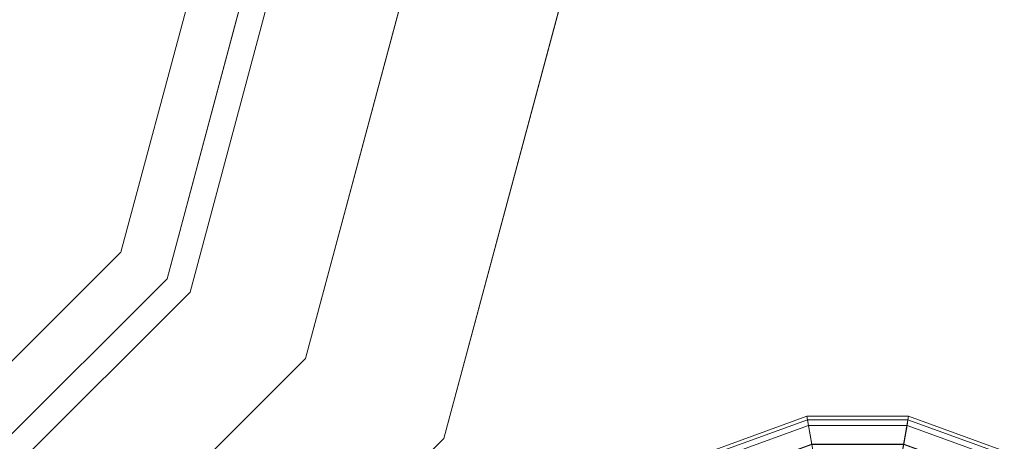
# Model space of a CAD drawing. Units: inches. Extents: x 375 to 1122, y 27 to 1069.
# Tile 44 of 155: x 715.392 to 719.94, y 300.305 to 302.255. Entities that reach past the tile are written whole.
import ezdxf

# ---------------------------------------------------------------- set-up
doc = ezdxf.new("R2010")
doc.units = ezdxf.units.IN
doc.layers.add('Furniture', color=30, linetype='Continuous', lineweight=18)

# ---------------------------------------------------------------- blocks, each defined once
blk = doc.blocks.new('A$C403C54AD')
for points in [[(1.15375, 0.87318, -0.02859), (1.15093, 0.87482, -0.03183), (1.1469, 0.86376, -0.03183), (1.15012, 0.8632, -0.02859)], [(1.15093, 0.87482, -0.03183), (1.18025, 0.85788, -0.02875), (1.18025, 0.85788, -0.02875), (1.1469, 0.86376, -0.03183)], [(1.15379, 0.87316, 0.13116), (1.15127, 0.87462, 0.11793), (1.1473, 0.86369, 0.11793), (1.15016, 0.86319, 0.13116)], [(1.15127, 0.87462, 0.11793), (1.15186, 0.87428, 0.08969), (1.14796, 0.86358, 0.08969), (1.1473, 0.86369, 0.11793)], [(1.15186, 0.87428, 0.08969), (1.1565, 0.8716, 0.07168), (1.15324, 0.86265, 0.07168), (1.14796, 0.86358, 0.08969)], [(1.15012, 0.8632, -0.02859), (1.1469, 0.86376, -0.03183), (1.1469, 0.852, -0.03183), (1.15012, 0.85257, -0.02859)], [(1.1469, 0.86376, -0.03183), (1.18025, 0.85788, -0.02875), (1.18025, 0.85788, -0.02875), (1.1469, 0.852, -0.03183)], [(1.15016, 0.86319, 0.13116), (1.1473, 0.86369, 0.11793), (1.1473, 0.85207, 0.11793), (1.15016, 0.85258, 0.13116)], [(1.1473, 0.86369, 0.11793), (1.14796, 0.86358, 0.08969), (1.14796, 0.85219, 0.08969), (1.1473, 0.85207, 0.11793)], [(1.14796, 0.86358, 0.08969), (1.15324, 0.86265, 0.07168), (1.15324, 0.85312, 0.07168), (1.14796, 0.85219, 0.08969)], [(1.1469, 0.852, -0.03183), (1.18025, 0.85788, -0.02875), (1.18025, 0.85788, -0.02875), (1.15093, 0.84095, -0.03183)], [(1.14796, 0.85219, 0.08969), (1.15324, 0.85312, 0.07168), (1.1565, 0.84417, 0.07168), (1.15186, 0.84149, 0.08969)], [(1.15012, 0.85257, -0.02859), (1.1469, 0.852, -0.03183), (1.15093, 0.84095, -0.03183), (1.15375, 0.84259, -0.02859)], [(1.15016, 0.85258, 0.13116), (1.1473, 0.85207, 0.11793), (1.15127, 0.84115, 0.11793), (1.15379, 0.84261, 0.13116)], [(1.1473, 0.85207, 0.11793), (1.14796, 0.85219, 0.08969), (1.15186, 0.84149, 0.08969), (1.15127, 0.84115, 0.11793)]]:
    blk.add_3dface(points)
at = {"linetype": 'ByBlock', "invisible_edges": 5}
for points in [[(1.14947, 0.81008, -0.00874), (1.14023, 0.79408, -0.00874), (1.0802, 0.81017, -0.00874), (1.0802, 0.82864, -0.00874)], [(1.13254, 0.78075, -0.02259), (1.14947, 0.81008, -0.01335), (1.0802, 0.82864, -0.01335), (1.0802, 0.79478, -0.02259)], [(1.14023, 0.79408, -0.00874), (1.131, 0.77809, -0.01489), (1.0802, 0.7917, -0.01489), (1.0802, 0.81017, -0.00874)], [(1.17085, 0.74244, -0.02259), (1.20017, 0.75938, -0.01335), (1.14947, 0.81008, -0.01335), (1.13254, 0.78075, -0.02259)], [(1.20017, 0.75938, -0.00874), (1.18418, 0.75014, -0.00874), (1.14023, 0.79408, -0.00874), (1.14947, 0.81008, -0.00874)], [(1.12792, 0.77276, -0.03183), (1.13254, 0.78075, -0.02259), (1.0802, 0.79478, -0.02259), (1.0802, 0.78554, -0.03183)], [(1.18418, 0.75014, -0.00874), (1.16818, 0.74091, -0.01489), (1.131, 0.77809, -0.01489), (1.14023, 0.79408, -0.00874)], [(1.131, 0.77809, -0.01489), (1.0802, 0.69011, -0.01489), (1.0802, 0.69011, -0.01489), (1.0802, 0.7917, -0.01489)], [(1.16285, 0.73783, -0.03183), (1.17085, 0.74244, -0.02259), (1.13254, 0.78075, -0.02259), (1.12792, 0.77276, -0.03183)], [(1.16818, 0.74091, -0.01489), (1.0802, 0.69011, -0.01489), (1.0802, 0.69011, -0.01489), (1.131, 0.77809, -0.01489)]]:
    blk.add_3dface(points, dxfattribs=at)
at = {"linetype": 'ByBlock'}
for points in [[(1.14947, 0.81008, -0.01335), (1.14947, 0.81008, -0.00874), (1.0802, 0.82864, -0.00874), (1.0802, 0.82864, -0.01335)], [(1.20017, 0.75938, -0.01335), (1.20017, 0.75938, -0.00874), (1.14947, 0.81008, -0.00874), (1.14947, 0.81008, -0.01335)]]:
    blk.add_3dface(points, dxfattribs=at)

msp = doc.modelspace()

# ---------------------------------------------------------------- block references
at = {"layer": 'Furniture', "xscale": 39.9918517141215, "yscale": 39.9918517141215, "zscale": 39.9918517141215, "rotation": 270}
msp.add_blockref('A$C403C54AD', (684.9549, 346.2875, 0.024), dxfattribs=at)

doc.saveas('drawing.dxf')
